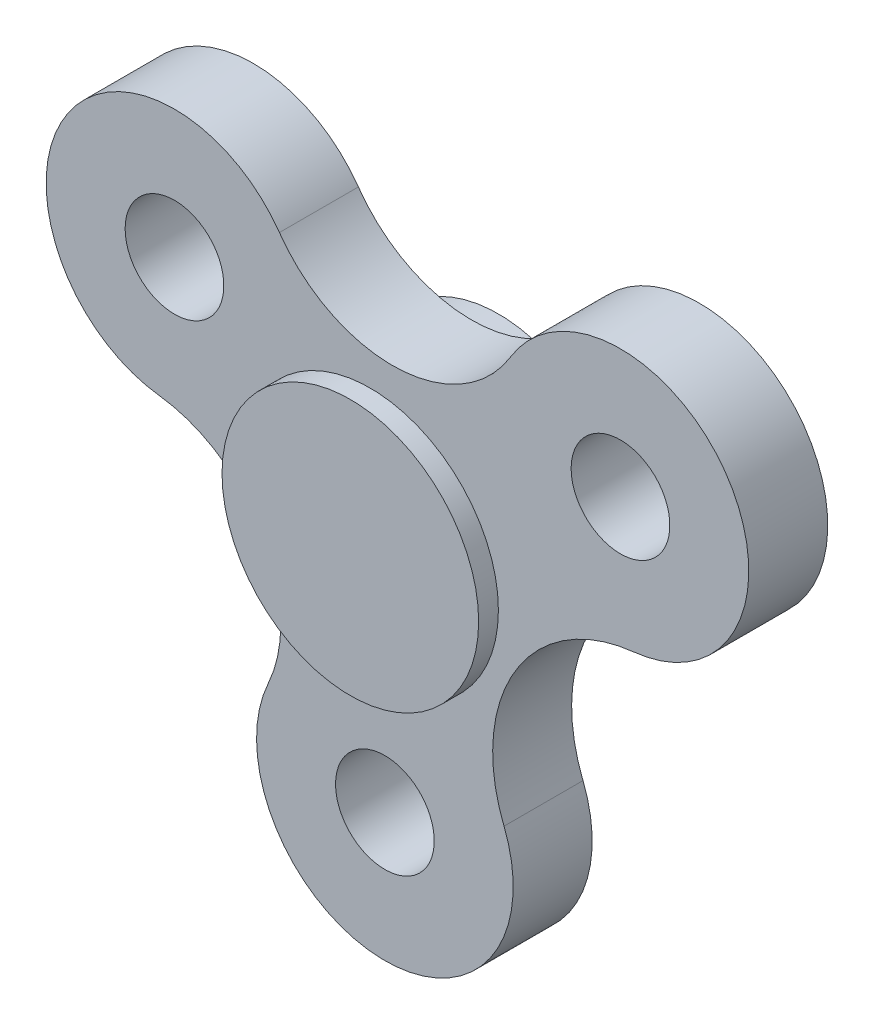
ISO-10303-21;
HEADER;
FILE_DESCRIPTION(('STEP AP214'),'2;1');
FILE_NAME('part.step','',(''),(''),'','','');
FILE_SCHEMA(('AUTOMOTIVE_DESIGN { 1 0 10303 214 1 1 1 1 }'));
ENDSEC;
DATA;
#1=APPLICATION_CONTEXT('core data for automotive mechanical design processes');
#2=APPLICATION_PROTOCOL_DEFINITION('international standard','automotive_design',2000,#1);
#3=PRODUCT_CONTEXT('',#1,'mechanical');
#4=PRODUCT('Part','Part','',(#3));
#5=PRODUCT_RELATED_PRODUCT_CATEGORY('part','',(#4));
#6=PRODUCT_DEFINITION_FORMATION('','',#4);
#7=PRODUCT_DEFINITION_CONTEXT('part definition',#1,'design');
#8=PRODUCT_DEFINITION('design','',#6,#7);
#9=PRODUCT_DEFINITION_SHAPE('','',#8);
#10=(LENGTH_UNIT() NAMED_UNIT(*) SI_UNIT(.MILLI.,.METRE.));
#11=(NAMED_UNIT(*) PLANE_ANGLE_UNIT() SI_UNIT($,.RADIAN.));
#12=(NAMED_UNIT(*) SI_UNIT($,.STERADIAN.) SOLID_ANGLE_UNIT());
#13=UNCERTAINTY_MEASURE_WITH_UNIT(LENGTH_MEASURE(1.E-05),#10,'distance_accuracy_value','');
#14=(GEOMETRIC_REPRESENTATION_CONTEXT(3) GLOBAL_UNCERTAINTY_ASSIGNED_CONTEXT((#13)) GLOBAL_UNIT_ASSIGNED_CONTEXT((#10,
#11,#12)) REPRESENTATION_CONTEXT('',''));
#15=CARTESIAN_POINT('',(0.,0.,0.));
#16=DIRECTION('',(0.,0.,1.));
#17=DIRECTION('',(1.,0.,0.));
#18=AXIS2_PLACEMENT_3D('',#15,#16,#17);
#19=CARTESIAN_POINT('',(0.,-25.,8.));
#20=DIRECTION('',(0.,0.,-1.));
#21=DIRECTION('',(-1.,0.,0.));
#22=AXIS2_PLACEMENT_3D('',#19,#20,#21);
#23=CYLINDRICAL_SURFACE('',#22,13.);
#24=CARTESIAN_POINT('',(0.,-25.,0.));
#25=DIRECTION('',(0.,0.,1.));
#26=DIRECTION('',(1.,0.,0.));
#27=AXIS2_PLACEMENT_3D('',#24,#25,#26);
#28=CIRCLE('',#27,13.);
#29=CARTESIAN_POINT('',(-11.8164757628733,-19.5805073535038,0.));
#30=VERTEX_POINT('',#29);
#31=CARTESIAN_POINT('',(12.0673020216918,-20.164690090876,0.));
#32=VERTEX_POINT('',#31);
#33=EDGE_CURVE('E133',#30,#32,#28,.T.);
#34=ORIENTED_EDGE('',*,*,#33,.T.);
#35=DIRECTION('',(0.,0.,-1.));
#36=VECTOR('',#35,1.);
#37=CARTESIAN_POINT('',(12.0673020216918,-20.164690090876,8.));
#38=LINE('',#37,#36);
#39=CARTESIAN_POINT('',(12.0673020216918,-20.164690090876,8.));
#40=VERTEX_POINT('',#39);
#41=EDGE_CURVE('E54',#40,#32,#38,.T.);
#42=ORIENTED_EDGE('',*,*,#41,.F.);
#43=CARTESIAN_POINT('',(0.,-25.,8.));
#44=DIRECTION('',(0.,0.,1.));
#45=DIRECTION('',(1.,0.,0.));
#46=AXIS2_PLACEMENT_3D('',#43,#44,#45);
#47=CIRCLE('',#46,13.);
#48=CARTESIAN_POINT('',(-11.8164757628733,-19.5805073535038,8.));
#49=VERTEX_POINT('',#48);
#50=EDGE_CURVE('E144',#49,#40,#47,.T.);
#51=ORIENTED_EDGE('',*,*,#50,.F.);
#52=DIRECTION('',(0.,0.,-1.));
#53=VECTOR('',#52,1.);
#54=CARTESIAN_POINT('',(-11.8164757628733,-19.5805073535038,8.));
#55=LINE('',#54,#53);
#56=EDGE_CURVE('E135',#49,#30,#55,.T.);
#57=ORIENTED_EDGE('',*,*,#56,.T.);
#58=EDGE_LOOP('',(#34,#42,#51,#57));
#59=FACE_BOUND('',#58,.T.);
#60=ADVANCED_FACE('F50',(#59),#23,.T.);
#61=CARTESIAN_POINT('',(26.9193660483895,-14.2135394334927,8.));
#62=DIRECTION('',(0.,0.,-1.));
#63=DIRECTION('',(-1.,0.,0.));
#64=AXIS2_PLACEMENT_3D('',#61,#62,#63);
#65=CYLINDRICAL_SURFACE('',#64,16.);
#66=CARTESIAN_POINT('',(26.9193660483895,-14.2135394334927,0.));
#67=DIRECTION('',(0.,0.,1.));
#68=DIRECTION('',(1.,0.,0.));
#69=AXIS2_PLACEMENT_3D('',#66,#67,#68);
#70=CIRCLE('',#69,16.);
#71=CARTESIAN_POINT('',(25.2349318858063,1.69754731606414,0.));
#72=VERTEX_POINT('',#71);
#73=EDGE_CURVE('E138',#32,#72,#70,.F.);
#74=ORIENTED_EDGE('',*,*,#73,.T.);
#75=DIRECTION('',(0.,0.,-1.));
#76=VECTOR('',#75,1.);
#77=CARTESIAN_POINT('',(25.2349318858063,1.69754731606414,8.));
#78=LINE('',#77,#76);
#79=CARTESIAN_POINT('',(25.2349318858063,1.69754731606414,8.));
#80=VERTEX_POINT('',#79);
#81=EDGE_CURVE('E149',#80,#72,#78,.T.);
#82=ORIENTED_EDGE('',*,*,#81,.F.);
#83=CARTESIAN_POINT('',(26.9193660483895,-14.2135394334927,8.));
#84=DIRECTION('',(0.,0.,1.));
#85=DIRECTION('',(1.,0.,0.));
#86=AXIS2_PLACEMENT_3D('',#83,#84,#85);
#87=CIRCLE('',#86,16.);
#88=EDGE_CURVE('E99',#40,#80,#87,.F.);
#89=ORIENTED_EDGE('',*,*,#88,.F.);
#90=ORIENTED_EDGE('',*,*,#41,.T.);
#91=EDGE_LOOP('',(#74,#82,#89,#90));
#92=FACE_BOUND('',#91,.T.);
#93=ADVANCED_FACE('F155',(#92),#65,.F.);
#94=CARTESIAN_POINT('',(23.8663291287076,14.6253053000791,8.));
#95=DIRECTION('',(0.,0.,-1.));
#96=DIRECTION('',(-1.,0.,0.));
#97=AXIS2_PLACEMENT_3D('',#94,#95,#96);
#98=CYLINDRICAL_SURFACE('',#97,13.);
#99=CARTESIAN_POINT('',(23.8663291287076,14.6253053000791,0.));
#100=DIRECTION('',(0.,0.,1.));
#101=DIRECTION('',(1.,0.,0.));
#102=AXIS2_PLACEMENT_3D('',#99,#100,#101);
#103=CIRCLE('',#102,13.);
#104=CARTESIAN_POINT('',(12.7433341704152,21.354271279916,0.));
#105=VERTEX_POINT('',#104);
#106=EDGE_CURVE('E139',#72,#105,#103,.T.);
#107=ORIENTED_EDGE('',*,*,#106,.T.);
#108=DIRECTION('',(0.,0.,-1.));
#109=VECTOR('',#108,1.);
#110=CARTESIAN_POINT('',(12.7433341704152,21.354271279916,8.));
#111=LINE('',#110,#109);
#112=CARTESIAN_POINT('',(12.7433341704152,21.354271279916,8.));
#113=VERTEX_POINT('',#112);
#114=EDGE_CURVE('E117',#113,#105,#111,.T.);
#115=ORIENTED_EDGE('',*,*,#114,.F.);
#116=CARTESIAN_POINT('',(23.8663291287076,14.6253053000791,8.));
#117=DIRECTION('',(0.,0.,1.));
#118=DIRECTION('',(1.,0.,0.));
#119=AXIS2_PLACEMENT_3D('',#116,#117,#118);
#120=CIRCLE('',#119,13.);
#121=EDGE_CURVE('E122',#80,#113,#120,.T.);
#122=ORIENTED_EDGE('',*,*,#121,.F.);
#123=ORIENTED_EDGE('',*,*,#81,.T.);
#124=EDGE_LOOP('',(#107,#115,#122,#123));
#125=FACE_BOUND('',#124,.T.);
#126=ADVANCED_FACE('F161',(#125),#98,.T.);
#127=CARTESIAN_POINT('',(0.764724215331145,28.6008500274327,8.));
#128=DIRECTION('',(0.,0.,-1.));
#129=DIRECTION('',(-1.,0.,0.));
#130=AXIS2_PLACEMENT_3D('',#127,#128,#129);
#131=CYLINDRICAL_SURFACE('',#130,14.);
#132=CARTESIAN_POINT('',(0.764724215331145,28.6008500274327,0.));
#133=DIRECTION('',(0.,0.,1.));
#134=DIRECTION('',(1.,0.,0.));
#135=AXIS2_PLACEMENT_3D('',#132,#133,#134);
#136=CIRCLE('',#135,14.);
#137=CARTESIAN_POINT('',(-10.6845423231343,20.5439091854521,0.));
#138=VERTEX_POINT('',#137);
#139=EDGE_CURVE('E113',#138,#105,#136,.T.);
#140=ORIENTED_EDGE('',*,*,#139,.F.);
#141=DIRECTION('',(0.,0.,-1.));
#142=VECTOR('',#141,1.);
#143=CARTESIAN_POINT('',(-10.6845423231343,20.5439091854521,8.));
#144=LINE('',#143,#142);
#145=CARTESIAN_POINT('',(-10.6845423231343,20.5439091854521,8.));
#146=VERTEX_POINT('',#145);
#147=EDGE_CURVE('E108',#146,#138,#144,.T.);
#148=ORIENTED_EDGE('',*,*,#147,.F.);
#149=CARTESIAN_POINT('',(0.764724215331145,28.6008500274327,8.));
#150=DIRECTION('',(0.,0.,1.));
#151=DIRECTION('',(1.,0.,0.));
#152=AXIS2_PLACEMENT_3D('',#149,#150,#151);
#153=CIRCLE('',#152,14.);
#154=EDGE_CURVE('E114',#146,#113,#153,.T.);
#155=ORIENTED_EDGE('',*,*,#154,.T.);
#156=ORIENTED_EDGE('',*,*,#114,.T.);
#157=EDGE_LOOP('',(#140,#148,#155,#156));
#158=FACE_BOUND('',#157,.T.);
#159=ADVANCED_FACE('F112',(#158),#131,.F.);
#160=CARTESIAN_POINT('',(-21.3160041088523,13.0624641178987,8.));
#161=DIRECTION('',(0.,0.,-1.));
#162=DIRECTION('',(-1.,0.,0.));
#163=AXIS2_PLACEMENT_3D('',#160,#161,#162);
#164=CYLINDRICAL_SURFACE('',#163,13.);
#165=CARTESIAN_POINT('',(-21.3160041088523,13.0624641178987,0.));
#166=DIRECTION('',(0.,0.,1.));
#167=DIRECTION('',(1.,0.,0.));
#168=AXIS2_PLACEMENT_3D('',#165,#166,#167);
#169=CIRCLE('',#168,13.);
#170=CARTESIAN_POINT('',(-22.8692186341301,0.155585152073354,0.));
#171=VERTEX_POINT('',#170);
#172=EDGE_CURVE('E82',#138,#171,#169,.T.);
#173=ORIENTED_EDGE('',*,*,#172,.T.);
#174=DIRECTION('',(0.,0.,-1.));
#175=VECTOR('',#174,1.);
#176=CARTESIAN_POINT('',(-22.8692186341301,0.155585152073354,8.));
#177=LINE('',#176,#175);
#178=CARTESIAN_POINT('',(-22.8692186341301,0.155585152073354,8.));
#179=VERTEX_POINT('',#178);
#180=EDGE_CURVE('E120',#179,#171,#177,.T.);
#181=ORIENTED_EDGE('',*,*,#180,.F.);
#182=CARTESIAN_POINT('',(-21.3160041088523,13.0624641178987,8.));
#183=DIRECTION('',(0.,0.,1.));
#184=DIRECTION('',(1.,0.,0.));
#185=AXIS2_PLACEMENT_3D('',#182,#183,#184);
#186=CIRCLE('',#185,13.);
#187=EDGE_CURVE('E119',#146,#179,#186,.T.);
#188=ORIENTED_EDGE('',*,*,#187,.F.);
#189=ORIENTED_EDGE('',*,*,#147,.T.);
#190=EDGE_LOOP('',(#173,#181,#188,#189));
#191=FACE_BOUND('',#190,.T.);
#192=ADVANCED_FACE('F116',(#191),#164,.T.);
#193=CARTESIAN_POINT('',(-24.5419111998139,-13.7441306572771,8.));
#194=DIRECTION('',(0.,0.,-1.));
#195=DIRECTION('',(-1.,0.,0.));
#196=AXIS2_PLACEMENT_3D('',#193,#194,#195);
#197=CYLINDRICAL_SURFACE('',#196,14.);
#198=CARTESIAN_POINT('',(-24.5419111998139,-13.7441306572771,0.));
#199=DIRECTION('',(0.,0.,1.));
#200=DIRECTION('',(1.,0.,0.));
#201=AXIS2_PLACEMENT_3D('',#198,#199,#200);
#202=CIRCLE('',#201,14.);
#203=EDGE_CURVE('E93',#171,#30,#202,.F.);
#204=ORIENTED_EDGE('',*,*,#203,.T.);
#205=ORIENTED_EDGE('',*,*,#56,.F.);
#206=CARTESIAN_POINT('',(-24.5419111998139,-13.7441306572771,8.));
#207=DIRECTION('',(0.,0.,1.));
#208=DIRECTION('',(1.,0.,0.));
#209=AXIS2_PLACEMENT_3D('',#206,#207,#208);
#210=CIRCLE('',#209,14.);
#211=EDGE_CURVE('E63',#179,#49,#210,.F.);
#212=ORIENTED_EDGE('',*,*,#211,.F.);
#213=ORIENTED_EDGE('',*,*,#180,.T.);
#214=EDGE_LOOP('',(#204,#205,#212,#213));
#215=FACE_BOUND('',#214,.T.);
#216=ADVANCED_FACE('F197',(#215),#197,.F.);
#217=CARTESIAN_POINT('',(0.,0.,8.));
#218=DIRECTION('',(0.,0.,1.));
#219=DIRECTION('',(1.,0.,0.));
#220=AXIS2_PLACEMENT_3D('',#217,#218,#219);
#221=PLANE('',#220);
#222=CARTESIAN_POINT('',(0.,0.,8.));
#223=DIRECTION('',(0.,0.,1.));
#224=DIRECTION('',(1.,0.,0.));
#225=AXIS2_PLACEMENT_3D('',#222,#223,#224);
#226=CIRCLE('',#225,10.);
#227=CARTESIAN_POINT('',(10.,0.,8.));
#228=VERTEX_POINT('',#227);
#229=EDGE_CURVE('E448',#228,#228,#226,.T.);
#230=ORIENTED_EDGE('',*,*,#229,.F.);
#231=EDGE_LOOP('',(#230));
#232=FACE_BOUND('',#231,.T.);
#233=ORIENTED_EDGE('',*,*,#50,.T.);
#234=ORIENTED_EDGE('',*,*,#88,.T.);
#235=ORIENTED_EDGE('',*,*,#121,.T.);
#236=ORIENTED_EDGE('',*,*,#154,.F.);
#237=ORIENTED_EDGE('',*,*,#187,.T.);
#238=ORIENTED_EDGE('',*,*,#211,.T.);
#239=EDGE_LOOP('',(#233,#234,#235,#236,#237,#238));
#240=FACE_BOUND('',#239,.T.);
#241=CARTESIAN_POINT('',(23.8663291287076,14.6253053000791,8.));
#242=DIRECTION('',(0.,0.,-1.));
#243=DIRECTION('',(-1.,0.,0.));
#244=AXIS2_PLACEMENT_3D('',#241,#242,#243);
#245=CIRCLE('',#244,5.);
#246=CARTESIAN_POINT('',(18.8663291287076,14.6253053000791,8.));
#247=VERTEX_POINT('',#246);
#248=EDGE_CURVE('E428',#247,#247,#245,.T.);
#249=ORIENTED_EDGE('',*,*,#248,.T.);
#250=EDGE_LOOP('',(#249));
#251=FACE_BOUND('',#250,.T.);
#252=CARTESIAN_POINT('',(-21.3160041088523,13.0624641178987,8.));
#253=DIRECTION('',(0.,0.,-1.));
#254=DIRECTION('',(-1.,0.,0.));
#255=AXIS2_PLACEMENT_3D('',#252,#253,#254);
#256=CIRCLE('',#255,5.);
#257=CARTESIAN_POINT('',(-26.3160041088523,13.0624641178987,8.));
#258=VERTEX_POINT('',#257);
#259=EDGE_CURVE('E425',#258,#258,#256,.T.);
#260=ORIENTED_EDGE('',*,*,#259,.T.);
#261=EDGE_LOOP('',(#260));
#262=FACE_BOUND('',#261,.T.);
#263=CARTESIAN_POINT('',(0.,-25.,8.));
#264=DIRECTION('',(0.,0.,-1.));
#265=DIRECTION('',(-1.,0.,0.));
#266=AXIS2_PLACEMENT_3D('',#263,#264,#265);
#267=CIRCLE('',#266,5.);
#268=CARTESIAN_POINT('',(-5.,-25.,8.));
#269=VERTEX_POINT('',#268);
#270=EDGE_CURVE('E411',#269,#269,#267,.T.);
#271=ORIENTED_EDGE('',*,*,#270,.T.);
#272=EDGE_LOOP('',(#271));
#273=FACE_BOUND('',#272,.T.);
#274=ADVANCED_FACE('F125',(#232,#240,#251,#262,#273),#221,.T.);
#275=CARTESIAN_POINT('',(0.,0.,0.));
#276=DIRECTION('',(0.,0.,1.));
#277=DIRECTION('',(1.,0.,0.));
#278=AXIS2_PLACEMENT_3D('',#275,#276,#277);
#279=PLANE('',#278);
#280=CARTESIAN_POINT('',(0.,0.,0.));
#281=DIRECTION('',(0.,0.,1.));
#282=DIRECTION('',(1.,0.,0.));
#283=AXIS2_PLACEMENT_3D('',#280,#281,#282);
#284=CIRCLE('',#283,11.);
#285=CARTESIAN_POINT('',(11.,0.,0.));
#286=VERTEX_POINT('',#285);
#287=EDGE_CURVE('E11',#286,#286,#284,.F.);
#288=ORIENTED_EDGE('',*,*,#287,.F.);
#289=EDGE_LOOP('',(#288));
#290=FACE_BOUND('',#289,.T.);
#291=ORIENTED_EDGE('',*,*,#33,.F.);
#292=ORIENTED_EDGE('',*,*,#203,.F.);
#293=ORIENTED_EDGE('',*,*,#172,.F.);
#294=ORIENTED_EDGE('',*,*,#139,.T.);
#295=ORIENTED_EDGE('',*,*,#106,.F.);
#296=ORIENTED_EDGE('',*,*,#73,.F.);
#297=EDGE_LOOP('',(#291,#292,#293,#294,#295,#296));
#298=FACE_BOUND('',#297,.T.);
#299=CARTESIAN_POINT('',(23.8663291287076,14.6253053000791,0.));
#300=DIRECTION('',(0.,0.,-1.));
#301=DIRECTION('',(-1.,0.,0.));
#302=AXIS2_PLACEMENT_3D('',#299,#300,#301);
#303=CIRCLE('',#302,5.);
#304=CARTESIAN_POINT('',(18.8663291287076,14.6253053000791,0.));
#305=VERTEX_POINT('',#304);
#306=EDGE_CURVE('E422',#305,#305,#303,.T.);
#307=ORIENTED_EDGE('',*,*,#306,.F.);
#308=EDGE_LOOP('',(#307));
#309=FACE_BOUND('',#308,.T.);
#310=CARTESIAN_POINT('',(-21.3160041088523,13.0624641178987,0.));
#311=DIRECTION('',(0.,0.,-1.));
#312=DIRECTION('',(-1.,0.,0.));
#313=AXIS2_PLACEMENT_3D('',#310,#311,#312);
#314=CIRCLE('',#313,5.);
#315=CARTESIAN_POINT('',(-26.3160041088523,13.0624641178987,0.));
#316=VERTEX_POINT('',#315);
#317=EDGE_CURVE('E420',#316,#316,#314,.T.);
#318=ORIENTED_EDGE('',*,*,#317,.F.);
#319=EDGE_LOOP('',(#318));
#320=FACE_BOUND('',#319,.T.);
#321=CARTESIAN_POINT('',(0.,-25.,0.));
#322=DIRECTION('',(0.,0.,-1.));
#323=DIRECTION('',(-1.,0.,0.));
#324=AXIS2_PLACEMENT_3D('',#321,#322,#323);
#325=CIRCLE('',#324,5.);
#326=CARTESIAN_POINT('',(-5.,-25.,0.));
#327=VERTEX_POINT('',#326);
#328=EDGE_CURVE('E418',#327,#327,#325,.T.);
#329=ORIENTED_EDGE('',*,*,#328,.F.);
#330=EDGE_LOOP('',(#329));
#331=FACE_BOUND('',#330,.T.);
#332=ADVANCED_FACE('F160',(#290,#298,#309,#320,#331),#279,.F.);
#333=CARTESIAN_POINT('',(0.,0.,9.5));
#334=DIRECTION('',(0.,0.,-1.));
#335=DIRECTION('',(-1.,0.,0.));
#336=AXIS2_PLACEMENT_3D('',#333,#334,#335);
#337=CYLINDRICAL_SURFACE('',#336,10.);
#338=CARTESIAN_POINT('',(0.,0.,9.5));
#339=DIRECTION('',(0.,0.,1.));
#340=DIRECTION('',(1.,0.,0.));
#341=AXIS2_PLACEMENT_3D('',#338,#339,#340);
#342=CIRCLE('',#341,10.);
#343=CARTESIAN_POINT('',(10.,0.,9.5));
#344=VERTEX_POINT('',#343);
#345=EDGE_CURVE('E140',#344,#344,#342,.T.);
#346=ORIENTED_EDGE('',*,*,#345,.F.);
#347=EDGE_LOOP('',(#346));
#348=FACE_BOUND('',#347,.T.);
#349=ORIENTED_EDGE('',*,*,#229,.T.);
#350=EDGE_LOOP('',(#349));
#351=FACE_BOUND('',#350,.T.);
#352=ADVANCED_FACE('F234',(#348,#351),#337,.T.);
#353=CARTESIAN_POINT('',(0.,0.,-1.5));
#354=DIRECTION('',(0.,0.,1.));
#355=DIRECTION('',(1.,0.,0.));
#356=AXIS2_PLACEMENT_3D('',#353,#354,#355);
#357=CYLINDRICAL_SURFACE('',#356,11.);
#358=CARTESIAN_POINT('',(0.,0.,-1.5));
#359=DIRECTION('',(0.,0.,-1.));
#360=DIRECTION('',(-1.,0.,0.));
#361=AXIS2_PLACEMENT_3D('',#358,#359,#360);
#362=CIRCLE('',#361,11.);
#363=CARTESIAN_POINT('',(-11.,0.,-1.5));
#364=VERTEX_POINT('',#363);
#365=EDGE_CURVE('E444',#364,#364,#362,.T.);
#366=ORIENTED_EDGE('',*,*,#365,.F.);
#367=EDGE_LOOP('',(#366));
#368=FACE_BOUND('',#367,.T.);
#369=ORIENTED_EDGE('',*,*,#287,.T.);
#370=EDGE_LOOP('',(#369));
#371=FACE_BOUND('',#370,.T.);
#372=ADVANCED_FACE('F255',(#368,#371),#357,.T.);
#373=CARTESIAN_POINT('',(0.,0.,-3.5));
#374=DIRECTION('',(0.,0.,1.));
#375=DIRECTION('',(1.,0.,0.));
#376=AXIS2_PLACEMENT_3D('',#373,#374,#375);
#377=CYLINDRICAL_SURFACE('',#376,13.);
#378=CARTESIAN_POINT('',(0.,0.,-3.5));
#379=DIRECTION('',(0.,0.,-1.));
#380=DIRECTION('',(-1.,0.,0.));
#381=AXIS2_PLACEMENT_3D('',#378,#379,#380);
#382=CIRCLE('',#381,13.);
#383=CARTESIAN_POINT('',(-13.,0.,-3.5));
#384=VERTEX_POINT('',#383);
#385=EDGE_CURVE('E439',#384,#384,#382,.T.);
#386=ORIENTED_EDGE('',*,*,#385,.F.);
#387=EDGE_LOOP('',(#386));
#388=FACE_BOUND('',#387,.T.);
#389=CARTESIAN_POINT('',(0.,0.,-1.5));
#390=DIRECTION('',(0.,0.,-1.));
#391=DIRECTION('',(-1.,0.,0.));
#392=AXIS2_PLACEMENT_3D('',#389,#390,#391);
#393=CIRCLE('',#392,13.);
#394=CARTESIAN_POINT('',(-13.,0.,-1.5));
#395=VERTEX_POINT('',#394);
#396=EDGE_CURVE('E440',#395,#395,#393,.T.);
#397=ORIENTED_EDGE('',*,*,#396,.T.);
#398=EDGE_LOOP('',(#397));
#399=FACE_BOUND('',#398,.T.);
#400=ADVANCED_FACE('F266',(#388,#399),#377,.T.);
#401=CARTESIAN_POINT('',(0.,0.,-3.5));
#402=DIRECTION('',(0.,0.,-1.));
#403=DIRECTION('',(-1.,0.,0.));
#404=AXIS2_PLACEMENT_3D('',#401,#402,#403);
#405=PLANE('',#404);
#406=ORIENTED_EDGE('',*,*,#385,.T.);
#407=EDGE_LOOP('',(#406));
#408=FACE_BOUND('',#407,.T.);
#409=ADVANCED_FACE('F279',(#408),#405,.T.);
#410=CARTESIAN_POINT('',(0.,0.,-1.5));
#411=DIRECTION('',(0.,0.,-1.));
#412=DIRECTION('',(-1.,0.,0.));
#413=AXIS2_PLACEMENT_3D('',#410,#411,#412);
#414=PLANE('',#413);
#415=ORIENTED_EDGE('',*,*,#365,.T.);
#416=EDGE_LOOP('',(#415));
#417=FACE_BOUND('',#416,.T.);
#418=ORIENTED_EDGE('',*,*,#396,.F.);
#419=EDGE_LOOP('',(#418));
#420=FACE_BOUND('',#419,.T.);
#421=ADVANCED_FACE('F287',(#417,#420),#414,.F.);
#422=CARTESIAN_POINT('',(0.,0.,11.5));
#423=DIRECTION('',(0.,0.,-1.));
#424=DIRECTION('',(-1.,0.,0.));
#425=AXIS2_PLACEMENT_3D('',#422,#423,#424);
#426=CYLINDRICAL_SURFACE('',#425,13.);
#427=CARTESIAN_POINT('',(0.,0.,11.5));
#428=DIRECTION('',(0.,0.,1.));
#429=DIRECTION('',(1.,0.,0.));
#430=AXIS2_PLACEMENT_3D('',#427,#428,#429);
#431=CIRCLE('',#430,13.);
#432=CARTESIAN_POINT('',(13.,0.,11.5));
#433=VERTEX_POINT('',#432);
#434=EDGE_CURVE('E432',#433,#433,#431,.T.);
#435=ORIENTED_EDGE('',*,*,#434,.F.);
#436=EDGE_LOOP('',(#435));
#437=FACE_BOUND('',#436,.T.);
#438=CARTESIAN_POINT('',(0.,0.,9.5));
#439=DIRECTION('',(0.,0.,1.));
#440=DIRECTION('',(1.,0.,0.));
#441=AXIS2_PLACEMENT_3D('',#438,#439,#440);
#442=CIRCLE('',#441,13.);
#443=CARTESIAN_POINT('',(13.,0.,9.5));
#444=VERTEX_POINT('',#443);
#445=EDGE_CURVE('E431',#444,#444,#442,.T.);
#446=ORIENTED_EDGE('',*,*,#445,.T.);
#447=EDGE_LOOP('',(#446));
#448=FACE_BOUND('',#447,.T.);
#449=ADVANCED_FACE('F305',(#437,#448),#426,.T.);
#450=CARTESIAN_POINT('',(0.,0.,11.5));
#451=DIRECTION('',(0.,0.,1.));
#452=DIRECTION('',(1.,0.,0.));
#453=AXIS2_PLACEMENT_3D('',#450,#451,#452);
#454=PLANE('',#453);
#455=ORIENTED_EDGE('',*,*,#434,.T.);
#456=EDGE_LOOP('',(#455));
#457=FACE_BOUND('',#456,.T.);
#458=ADVANCED_FACE('F314',(#457),#454,.T.);
#459=CARTESIAN_POINT('',(0.,0.,9.5));
#460=DIRECTION('',(0.,0.,1.));
#461=DIRECTION('',(1.,0.,0.));
#462=AXIS2_PLACEMENT_3D('',#459,#460,#461);
#463=PLANE('',#462);
#464=ORIENTED_EDGE('',*,*,#345,.T.);
#465=EDGE_LOOP('',(#464));
#466=FACE_BOUND('',#465,.T.);
#467=ORIENTED_EDGE('',*,*,#445,.F.);
#468=EDGE_LOOP('',(#467));
#469=FACE_BOUND('',#468,.T.);
#470=ADVANCED_FACE('F324',(#466,#469),#463,.F.);
#471=CARTESIAN_POINT('',(23.8663291287076,14.6253053000791,8.));
#472=DIRECTION('',(0.,0.,-1.));
#473=DIRECTION('',(-1.,0.,0.));
#474=AXIS2_PLACEMENT_3D('',#471,#472,#473);
#475=CYLINDRICAL_SURFACE('',#474,5.);
#476=ORIENTED_EDGE('',*,*,#248,.F.);
#477=EDGE_LOOP('',(#476));
#478=FACE_BOUND('',#477,.T.);
#479=ORIENTED_EDGE('',*,*,#306,.T.);
#480=EDGE_LOOP('',(#479));
#481=FACE_BOUND('',#480,.T.);
#482=ADVANCED_FACE('F337',(#478,#481),#475,.F.);
#483=CARTESIAN_POINT('',(-21.3160041088523,13.0624641178987,8.));
#484=DIRECTION('',(0.,0.,-1.));
#485=DIRECTION('',(-1.,0.,0.));
#486=AXIS2_PLACEMENT_3D('',#483,#484,#485);
#487=CYLINDRICAL_SURFACE('',#486,5.);
#488=ORIENTED_EDGE('',*,*,#259,.F.);
#489=EDGE_LOOP('',(#488));
#490=FACE_BOUND('',#489,.T.);
#491=ORIENTED_EDGE('',*,*,#317,.T.);
#492=EDGE_LOOP('',(#491));
#493=FACE_BOUND('',#492,.T.);
#494=ADVANCED_FACE('F363',(#490,#493),#487,.F.);
#495=CARTESIAN_POINT('',(0.,-25.,8.));
#496=DIRECTION('',(0.,0.,-1.));
#497=DIRECTION('',(-1.,0.,0.));
#498=AXIS2_PLACEMENT_3D('',#495,#496,#497);
#499=CYLINDRICAL_SURFACE('',#498,5.);
#500=ORIENTED_EDGE('',*,*,#270,.F.);
#501=EDGE_LOOP('',(#500));
#502=FACE_BOUND('',#501,.T.);
#503=ORIENTED_EDGE('',*,*,#328,.T.);
#504=EDGE_LOOP('',(#503));
#505=FACE_BOUND('',#504,.T.);
#506=ADVANCED_FACE('F375',(#502,#505),#499,.F.);
#507=CLOSED_SHELL('',(#60,#93,#126,#159,#192,#216,#274,#332,#352,#372,#400,#409,#421,#449,#458,
#470,#482,#494,#506));
#508=MANIFOLD_SOLID_BREP('B2',#507);
#509=ADVANCED_BREP_SHAPE_REPRESENTATION('',(#18,#508),#14);
#510=SHAPE_DEFINITION_REPRESENTATION(#9,#509);
ENDSEC;
END-ISO-10303-21;
